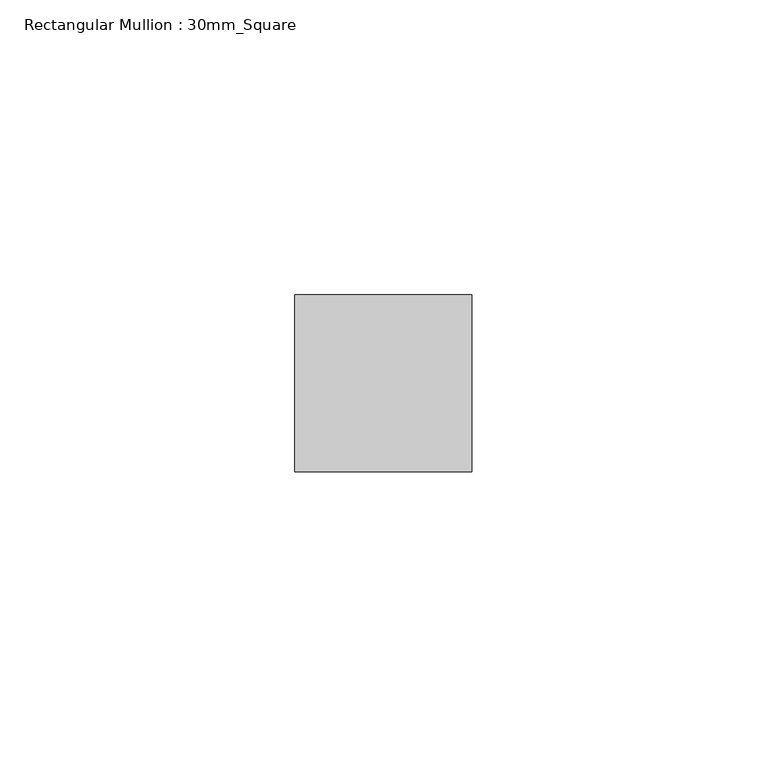
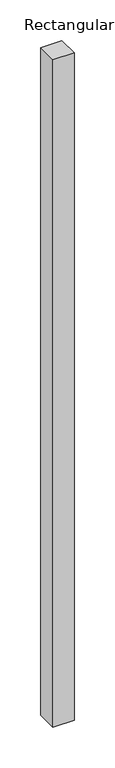
"""IFC4 building model written with IfcOpenShell, lengths in millimetres: member geometry, Rectangular Mullion : 30mm_Square."""

from ifc_helpers import new_model, si_unit, frame, origin, place, context, project, spatial, polyline, outline, extrude, source, transform, mapped, element, save


def rectangular_mullion_30mm_square_d725415c(model_context):
    return source(origin(), model_context, "Body", "SweptSolid", [
        extrude(outline(polyline([(0.0, 15.0), (0.0, -15.0), (-30.0, -15.0), (-30.0, 15.0), (0.0, 15.0)])), frame((0.0, 0.0, -999.4800296), z_axis=(0.0, 0.0, 1.0), x_axis=(1.0, 0.0, 0.0)), (0.0, 0.0, 1.0), 999.4800296),
    ])


if __name__ == "__main__":
    model = new_model("IFC4")
    model_context = context("Model", 3, world=origin())
    ifc_project = project(units=[si_unit("LENGTHUNIT", "METRE", prefix="MILLI")], contexts=[model_context])
    site = spatial("IfcSite", under=ifc_project)
    building = spatial("IfcBuilding", under=site)
    placement = place(None, origin())
    rectangular_mullion_30mm_square_shape = rectangular_mullion_30mm_square_d725415c(model_context)
    element("IfcMember", 1, ObjectType="Rectangular Mullion : 30mm_Square", at=placement, inside=building, context=model_context, shape_type="MappedRepresentation", body=[
        mapped(rectangular_mullion_30mm_square_shape, transform((0.0, 0.0, 0.0), x_axis=(1.0, 0.0, 0.0), y_axis=(0.0, 1.0, 0.0), z_axis=(0.0, 0.0, 1.0))),
    ])
    save(model, "model.ifc")

# Revit data of these elements
# Type "Rectangular Mullion : 30mm_Square"
#   Keynote = "H11"
#   built-in parameter 1007304 = 0.0984252 (stored number, unit not read)
#   built-in parameter 1007301 = 0.0492126 (stored number, unit not read)
#   built-in parameter 1007300 = 0.0492126 (stored number, unit not read)
# Element 1 (IfcMember, "Rectangular Mullion : 30mm_Square")
#   Materials on its faces: "Aluminium"
# Materials
#   "Aluminium": class "Metal", colour RGB 247 247 247, transparency 0, Description = "Aluminium 6061", Cost = 0
